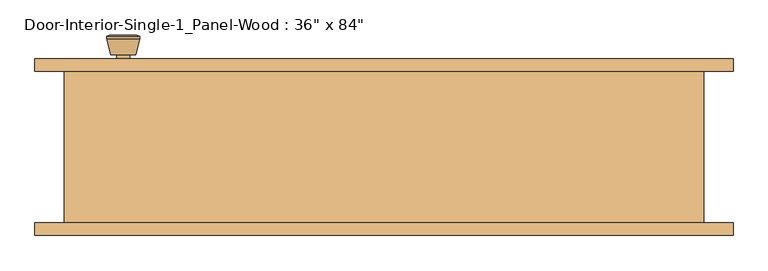
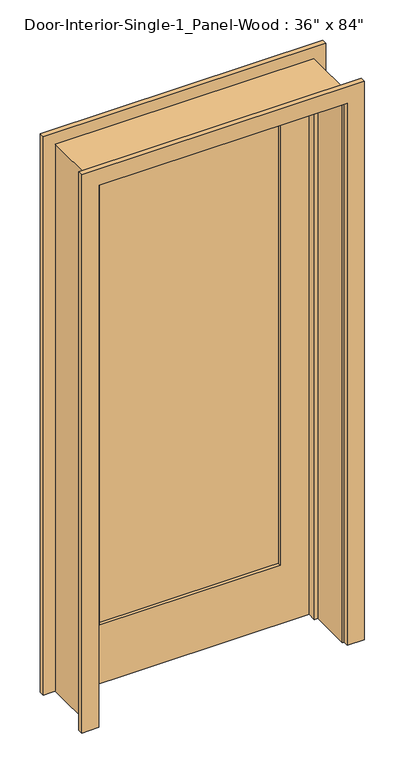
"""IFC4 building model written with IfcOpenShell, lengths in millimetres: door geometry."""

from ifc_helpers import new_model, si_unit, point, frame, frame_2d, origin, place, context, project, spatial, polyline, circle_curve, trimmed, segment, composite_curve, outline, extrude, faceted_brep, source, transform, mapped, element, save
from ifc_brep_helpers import plane_surface, cylinder_surface, revolved_surface, advanced_brep


def door_3b97b8e7(model_context):
    return source(origin(), model_context, "Body", "SolidModel", [
        advanced_brep(
        [(-393.7, 70.2, 914.4), (-383.7, 70.2, 914.4), (-403.7, 70.2, 914.4), (-373.2241324, 21.2, 914.4), (-393.7, 21.2, 914.4), (-414.1758676, 21.2, 914.4), (-368.7, 23.0278681, 914.4), (-418.7, 23.0278681, 914.4), (-368.7, 26.4915463, 914.4), (-418.7, 26.4915463, 914.4), (-375.063764, 51.2, 914.4), (-412.336236, 51.2, 914.4), (-383.7, 51.2, 914.4), (-403.7, 51.2, 914.4)],
        [
            (0, 1),
            (1, 2, circle_curve(frame((-393.7, 70.2, 914.4), z_axis=(0.0, 1.0, 0.0), x_axis=(-1.0, 0.0, 0.0)), 10.0)),
            (2, 0),
            (2, 1, circle_curve(frame((-393.7, 70.2, 914.4), z_axis=(0.0, 1.0, 0.0), x_axis=(-1.0, 0.0, 0.0)), 10.0)),
            (3, 4),
            (4, 5),
            (5, 3, circle_curve(frame((-393.7, 21.2, 914.4), z_axis=(0.0, -1.0, 0.0), x_axis=(-1.0, 0.0, 0.0)), 20.4758676)),
            (3, 5, circle_curve(frame((-393.7, 21.2, 914.4), z_axis=(0.0, -1.0, 0.0), x_axis=(-1.0, 0.0, 0.0)), 20.4758676)),
            (6, 3),
            (5, 7),
            (7, 6, circle_curve(frame((-393.7, 23.0278681, 914.4), z_axis=(0.0, -1.0, 0.0), x_axis=(-1.0, 0.0, 0.0)), 25.0)),
            (6, 7, circle_curve(frame((-393.7, 23.0278681, 914.4), z_axis=(0.0, -1.0, 0.0), x_axis=(-1.0, 0.0, 0.0)), 25.0)),
            (8, 6),
            (7, 9),
            (9, 8, circle_curve(frame((-393.7, 26.4915463, 914.4), z_axis=(0.0, -1.0, 0.0), x_axis=(-1.0, 0.0, 0.0)), 25.0)),
            (8, 9, circle_curve(frame((-393.7, 26.4915463, 914.4), z_axis=(0.0, -1.0, 0.0), x_axis=(-1.0, 0.0, 0.0)), 25.0)),
            (10, 8),
            (9, 11),
            (11, 10, circle_curve(frame((-393.7, 51.2, 914.4), z_axis=(0.0, -1.0, 0.0), x_axis=(-1.0, 0.0, 0.0)), 18.636236)),
            (10, 11, circle_curve(frame((-393.7, 51.2, 914.4), z_axis=(0.0, -1.0, 0.0), x_axis=(-1.0, 0.0, 0.0)), 18.636236)),
            (12, 10),
            (11, 13),
            (13, 12, circle_curve(frame((-393.7, 51.2, 914.4), z_axis=(0.0, -1.0, 0.0), x_axis=(-1.0, 0.0, 0.0)), 10.0)),
            (12, 13, circle_curve(frame((-393.7, 51.2, 914.4), z_axis=(0.0, -1.0, 0.0), x_axis=(-1.0, 0.0, 0.0)), 10.0)),
            (1, 12),
            (13, 2),
        ],
        [
            plane_surface(frame((-393.7, 70.2, 914.4), z_axis=(0.0, 1.0, 0.0), x_axis=(-1.0, 0.0, 0.0))),
            plane_surface(frame((-393.7, 21.2, 914.4), z_axis=(0.0, -1.0, 0.0), x_axis=(-1.0, 0.0, 0.0))),
            revolved_surface(polyline([(-414.1758676, 21.2, 914.4), (-418.7, 23.0278681, 914.4)]), (-393.7, 70.2, 914.4), (0.0, 1.0, 0.0)),
            cylinder_surface(frame((-393.7, 70.2, 914.4), z_axis=(0.0, 1.0, 0.0), x_axis=(-1.0, 0.0, 0.0)), 25.0),
            revolved_surface(polyline([(-418.7, 26.4915463, 914.4), (-412.336236, 51.2, 914.4)]), (-393.7, 70.2, 914.4), (0.0, 1.0, 0.0)),
            plane_surface(frame((-393.7, 51.2, 914.4), z_axis=(0.0, 1.0, 0.0), x_axis=(-1.0, 0.0, 0.0))),
            cylinder_surface(frame((-393.7, 70.2, 914.4), z_axis=(0.0, 1.0, 0.0), x_axis=(-1.0, 0.0, 0.0)), 10.0),
        ],
        [
            (0, [[1, 2, 3]]),
            (0, [[-3, 4, -1]]),
            (1, [[5, 6, 7]]),
            (1, [[-6, -5, 8]]),
            (2, [[9, -7, 10, 11]]),
            (2, [[-10, -8, -9, 12]]),
            (3, [[13, -11, 14, 15]]),
            (3, [[-14, -12, -13, 16]]),
            (4, [[17, -15, 18, 19]]),
            (4, [[-18, -16, -17, 20]]),
            (5, [[21, -19, 22, 23]]),
            (5, [[-22, -20, -21, 24]]),
            (6, [[25, -23, 26, -2]]),
            (6, [[-26, -24, -25, -4]]),
        ],
    ),
        extrude(outline(composite_curve([segment(trimmed(circle_curve(frame_2d((914.4, -393.7)), 30.0), [point((914.4, -423.7))], [point((914.4, -363.7))], False, "CARTESIAN"), True, "CONTINUOUS"), segment(trimmed(circle_curve(frame_2d((914.4, -393.7)), 30.0), [point((914.4, -363.7))], [point((914.4, -423.7))], False, "CARTESIAN"), True, "CONTINUOUS")], self_intersect=False)), frame((0.0, 70.2, 0.0), z_axis=(0.0, 1.0, 0.0), x_axis=(0.0, 0.0, 1.0)), (0.0, 0.0, 1.0), 6.0),
        advanced_brep(
        [(-393.7, 117.125, 914.4), (-403.7, 117.125, 914.4), (-383.7, 117.125, 914.4), (-373.2241324, 166.125, 914.4), (-414.1758676, 166.125, 914.4), (-393.7, 166.125, 914.4), (-368.7, 164.2971319, 914.4), (-418.7, 164.2971319, 914.4), (-368.7, 160.8334537, 914.4), (-418.7, 160.8334537, 914.4), (-375.063764, 136.125, 914.4), (-412.336236, 136.125, 914.4), (-383.7, 136.125, 914.4), (-403.7, 136.125, 914.4)],
        [
            (0, 1),
            (1, 2, circle_curve(frame((-393.7, 117.125, 914.4), z_axis=(0.0, -1.0, 0.0), x_axis=(-1.0, 0.0, 0.0)), 10.0)),
            (2, 0),
            (2, 1, circle_curve(frame((-393.7, 117.125, 914.4), z_axis=(0.0, -1.0, 0.0), x_axis=(-1.0, 0.0, 0.0)), 10.0)),
            (3, 4, circle_curve(frame((-393.7, 166.125, 914.4), z_axis=(0.0, 1.0, 0.0), x_axis=(-1.0, 0.0, 0.0)), 20.4758676)),
            (4, 5),
            (5, 3),
            (4, 3, circle_curve(frame((-393.7, 166.125, 914.4), z_axis=(0.0, 1.0, 0.0), x_axis=(-1.0, 0.0, 0.0)), 20.4758676)),
            (6, 7, circle_curve(frame((-393.7, 164.2971319, 914.4), z_axis=(0.0, 1.0, 0.0), x_axis=(-1.0, 0.0, 0.0)), 25.0)),
            (7, 4),
            (3, 6),
            (7, 6, circle_curve(frame((-393.7, 164.2971319, 914.4), z_axis=(0.0, 1.0, 0.0), x_axis=(-1.0, 0.0, 0.0)), 25.0)),
            (8, 9, circle_curve(frame((-393.7, 160.8334537, 914.4), z_axis=(0.0, 1.0, 0.0), x_axis=(-1.0, 0.0, 0.0)), 25.0)),
            (9, 7),
            (6, 8),
            (9, 8, circle_curve(frame((-393.7, 160.8334537, 914.4), z_axis=(0.0, 1.0, 0.0), x_axis=(-1.0, 0.0, 0.0)), 25.0)),
            (10, 11, circle_curve(frame((-393.7, 136.125, 914.4), z_axis=(0.0, 1.0, 0.0), x_axis=(-1.0, 0.0, 0.0)), 18.636236)),
            (11, 9),
            (8, 10),
            (11, 10, circle_curve(frame((-393.7, 136.125, 914.4), z_axis=(0.0, 1.0, 0.0), x_axis=(-1.0, 0.0, 0.0)), 18.636236)),
            (12, 13, circle_curve(frame((-393.7, 136.125, 914.4), z_axis=(0.0, 1.0, 0.0), x_axis=(-1.0, 0.0, 0.0)), 10.0)),
            (13, 11),
            (10, 12),
            (13, 12, circle_curve(frame((-393.7, 136.125, 914.4), z_axis=(0.0, 1.0, 0.0), x_axis=(-1.0, 0.0, 0.0)), 10.0)),
            (1, 13),
            (12, 2),
        ],
        [
            plane_surface(frame((-393.7, 117.125, 914.4), z_axis=(0.0, -1.0, 0.0), x_axis=(-1.0, 0.0, 0.0))),
            plane_surface(frame((-393.7, 166.125, 914.4), z_axis=(0.0, 1.0, 0.0), x_axis=(-1.0, 0.0, 0.0))),
            revolved_surface(polyline([(-414.1758676, 166.125, 914.4), (-418.7, 164.2971319, 914.4)]), (-393.7, 117.125, 914.4), (0.0, -1.0, 0.0)),
            cylinder_surface(frame((-393.7, 117.125, 914.4), z_axis=(0.0, -1.0, 0.0), x_axis=(-1.0, 0.0, 0.0)), 25.0),
            revolved_surface(polyline([(-418.7, 160.8334537, 914.4), (-412.336236, 136.125, 914.4)]), (-393.7, 117.125, 914.4), (0.0, -1.0, 0.0)),
            plane_surface(frame((-393.7, 136.125, 914.4), z_axis=(0.0, -1.0, 0.0), x_axis=(-1.0, 0.0, 0.0))),
            cylinder_surface(frame((-393.7, 117.125, 914.4), z_axis=(0.0, -1.0, 0.0), x_axis=(-1.0, 0.0, 0.0)), 10.0),
        ],
        [
            (0, [[1, 2, 3]]),
            (0, [[-3, 4, -1]]),
            (1, [[5, 6, 7]]),
            (1, [[8, -7, -6]]),
            (2, [[9, 10, -5, 11]]),
            (2, [[12, -11, -8, -10]]),
            (3, [[13, 14, -9, 15]]),
            (3, [[16, -15, -12, -14]]),
            (4, [[17, 18, -13, 19]]),
            (4, [[20, -19, -16, -18]]),
            (5, [[21, 22, -17, 23]]),
            (5, [[24, -23, -20, -22]]),
            (6, [[-2, 25, -21, 26]]),
            (6, [[-4, -26, -24, -25]]),
        ],
    ),
        extrude(outline(composite_curve([segment(trimmed(circle_curve(frame_2d((914.4, -393.7)), 30.0), [point((914.4, -423.7))], [point((914.4, -363.7))], False, "CARTESIAN"), True, "CONTINUOUS"), segment(trimmed(circle_curve(frame_2d((914.4, -393.7)), 30.0), [point((914.4, -363.7))], [point((914.4, -423.7))], False, "CARTESIAN"), True, "CONTINUOUS")], self_intersect=False)), frame((0.0, 111.125, 0.0), z_axis=(0.0, 1.0, 0.0), x_axis=(0.0, 0.0, 1.0)), (0.0, 0.0, 1.0), 6.0),
        faceted_brep([(482.6, 111.125, 0.0), (482.6, -117.475, 0.0), (457.2, -117.475, 0.0), (457.2, 41.275, 0.0), (444.5, 41.275, 0.0), (444.5, 76.2, 0.0), (457.2, 76.2, 0.0), (457.2, 111.125, 0.0), (482.6, 111.125, 2159.0), (482.6, -117.475, 2159.0), (-482.6, -117.475, 2159.0), (-482.6, -117.475, 0.0), (-457.2, -117.475, 0.0), (-457.2, -117.475, 2133.6), (457.2, -117.475, 2133.6), (457.2, 41.275, 2133.6), (-457.2, 41.275, 2133.6), (-457.2, 41.275, 0.0), (-444.5, 41.275, 0.0), (-444.5, 41.275, 2120.9), (444.5, 41.275, 2120.9), (444.5, 76.2, 2120.9), (-444.5, 76.2, 2120.9), (-444.5, 76.2, 0.0), (-457.2, 76.2, 0.0), (-457.2, 76.2, 2133.6), (457.2, 76.2, 2133.6), (457.2, 111.125, 2133.6), (-457.2, 111.125, 2133.6), (-457.2, 111.125, 0.0), (-482.6, 111.125, 0.0), (-482.6, 111.125, 2159.0)], [[[0, 1, 2, 3, 4, 5, 6, 7]], [[1, 0, 8, 9]], [[2, 1, 9, 10, 11, 12, 13, 14]], [[3, 2, 14, 15]], [[4, 3, 15, 16, 17, 18, 19, 20]], [[5, 4, 20, 21]], [[6, 5, 21, 22, 23, 24, 25, 26]], [[7, 6, 26, 27]], [[0, 7, 27, 28, 29, 30, 31, 8]], [[9, 8, 31, 10]], [[15, 14, 13, 16]], [[21, 20, 19, 22]], [[27, 26, 25, 28]], [[30, 29, 24, 23, 18, 17, 12, 11]], [[10, 31, 30, 11]], [[16, 13, 12, 17]], [[22, 19, 18, 23]], [[28, 25, 24, 29]]]),
        extrude(outline(polyline([(2133.6, -457.2), (0.0, -457.2), (0.0, 457.2), (2133.6, 457.2), (2133.6, -457.2)]), holes=[polyline([(2014.5375, -336.55), (2014.5375, 336.55), (231.775, 336.55), (231.775, -336.55), (2014.5375, -336.55)])]), frame((0.0, 76.2, 0.0), z_axis=(0.0, 1.0, 0.0), x_axis=(0.0, 0.0, 1.0)), (0.0, 0.0, 1.0), 34.925),
        extrude(outline(polyline([(336.55, 87.8416667), (-336.55, 87.8416667), (-336.55, 99.4833333), (336.55, 99.4833333), (336.55, 87.8416667)])), frame((0.0, 0.0, 231.775), z_axis=(0.0, 0.0, 1.0), x_axis=(1.0, 0.0, 0.0)), (0.0, 0.0, 1.0), 1782.7625),
        extrude(outline(polyline([(0.0, 463.55), (0.0, 527.05), (2203.45, 527.05), (2203.45, -527.05), (0.0, -527.05), (0.0, -463.55), (2139.95, -463.55), (2139.95, 463.55), (0.0, 463.55)])), frame((0.0, 111.125, 0.0), z_axis=(0.0, 1.0, 0.0), x_axis=(0.0, 0.0, 1.0)), (0.0, 0.0, 1.0), 19.05),
        extrude(outline(polyline([(0.0, 463.55), (0.0, 527.05), (2203.45, 527.05), (2203.45, -527.05), (0.0, -527.05), (0.0, -463.55), (2139.95, -463.55), (2139.95, 463.55), (0.0, 463.55)])), frame((0.0, -136.525, 0.0), z_axis=(0.0, 1.0, 0.0), x_axis=(0.0, 0.0, 1.0)), (0.0, 0.0, 1.0), 19.05),
    ])


if __name__ == "__main__":
    model = new_model("IFC4")
    model_context = context("Model", 3, world=origin())
    ifc_project = project(units=[si_unit("LENGTHUNIT", "METRE", prefix="MILLI")], contexts=[model_context])
    site = spatial("IfcSite", under=ifc_project)
    building = spatial("IfcBuilding", under=site)
    placement = place(None, origin())
    door_shape = door_3b97b8e7(model_context)
    element("IfcDoor", 1, ObjectType="Door-Interior-Single-1_Panel-Wood : 36\" x 84\"", at=placement, inside=building, context=model_context, shape_type="MappedRepresentation", body=[
        mapped(door_shape, transform((0.0, 0.0, 0.0), x_axis=(1.0, 0.0, 0.0), y_axis=(0.0, 1.0, 0.0), z_axis=(0.0, 0.0, 1.0))),
    ])
    save(model, "model.ifc")

# Revit data of these elements
# Type "Door-Interior-Single-1_Panel-Wood : 36\" x 84\""
#   Type Mark = "17"
#   Assembly Code = "C1020300"
#   Analytic Construction = "Wooden"
#   Top Rail = 0' - 4 11/16"
#   Thickness = 0' - 1 3/8"
#   Thermal Resistance (R) = 2.5876 (h·ft²·°F)/BTU
#   Swing Angle [instance default] = 90.00°
#   Stiles = 0' - 4 3/4"
#   Rough Width = 3' - 2"
#   Rough Height = 7' - 1"
#   Height = 7' - 0"
#   Width = 3' - 0"
#   Heat Transfer Coefficient (U) = 0.3865 BTU/(h·ft²·°F)
#   Bottom Rail = 0' - 9 1/8"
#   Trim Material = Cherry
#   Panel Material = Cherry
#   Frame Material = Cherry
#   Door Handle Material = Aluminum
#   Visual Light Transmittance = 0
#   Solar Heat Gain Coefficient = 0
#   Wall Closure = (empty or 0)
#   Function = (empty or 0)
# Element 1 (IfcDoor, "Door-Interior-Single-1_Panel-Wood : 36\" x 84\"")
#   Materials on its faces: "Cherry", "Aluminum"
# Materials
#   "Cherry": class "Wood", colour RGB 226 177 128, transparency 0, Description = "Prunus Serotina", Cost = 0
#   "Aluminum": class "Metal", colour RGB 247 247 247, transparency 0, Description = "Aluminum 6061", Cost = 0
